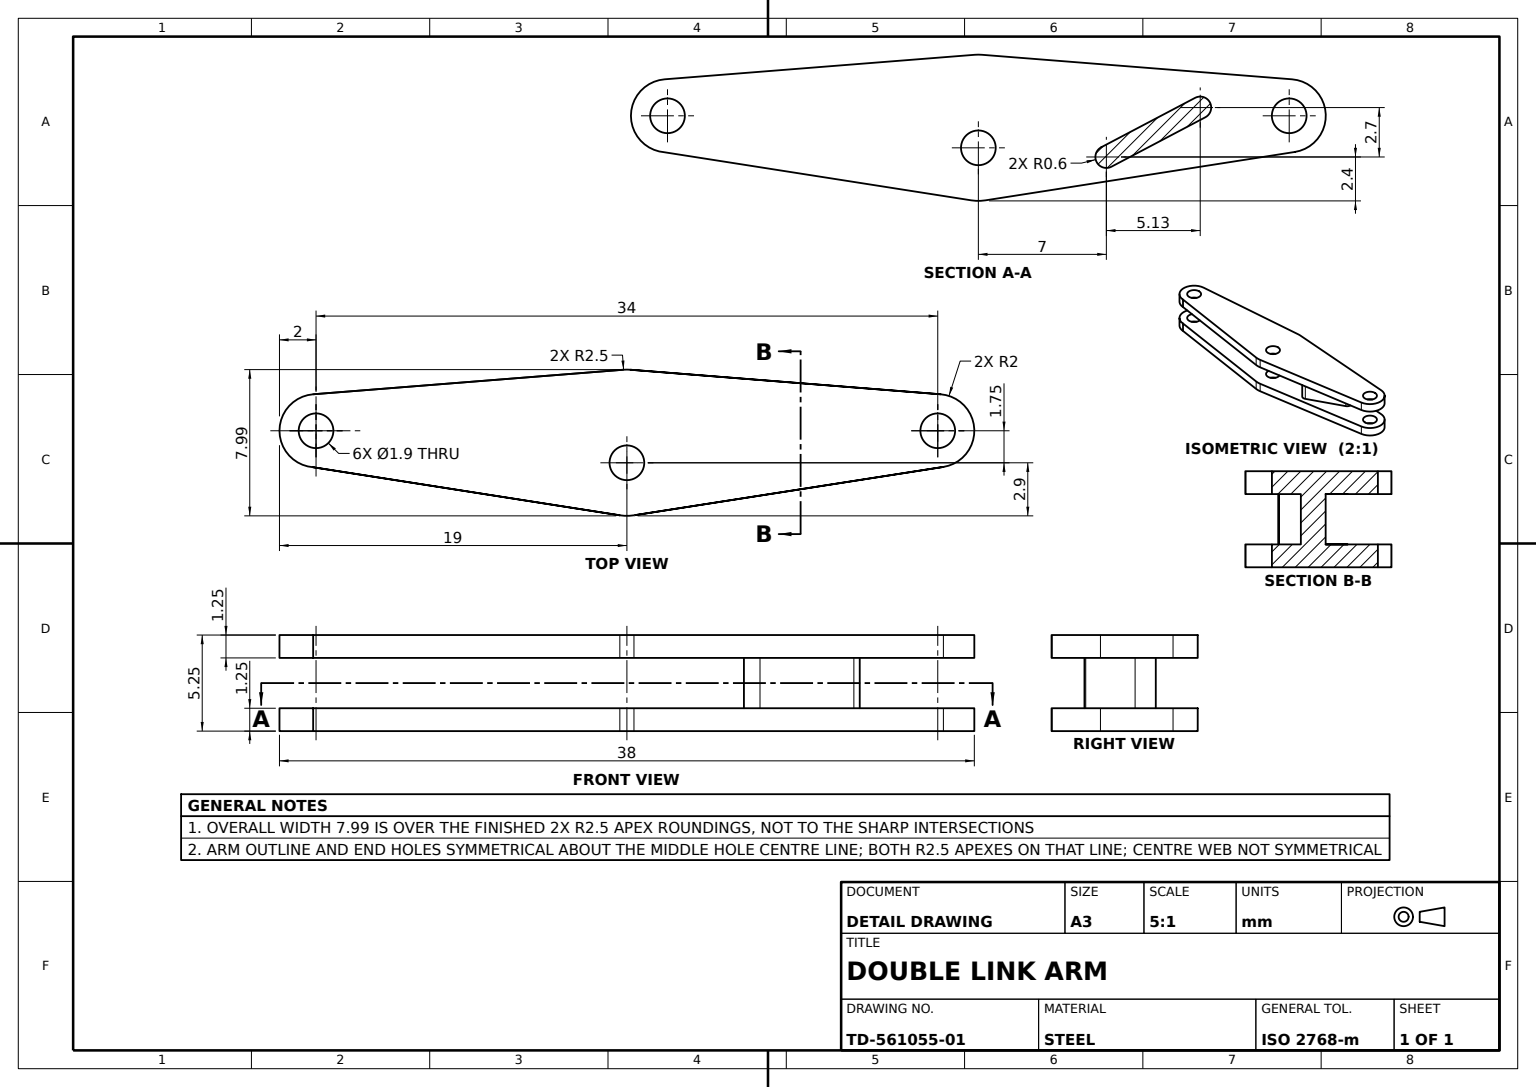
SolidWorks part; units mm, degrees
material "Plain Carbon Steel"
ref_plane "Front Plane" through (0, 0, 0) normal (0, 0, 1) x (1, 0, 0)
ref_plane "Top Plane" through (0, 0, 0) normal (0, 1, 0) x (1, 0, 0)
ref_plane "Right Plane" through (0, 0, 0) normal (1, 0, 0) x (0, 0, -1)
sketch "Arm Profile Sketch" plane through (0, 0, 0) normal (0, 1, 0) x (1, 0, 0)
  line L0 (17, 0) -> (-17, 0) construction
  line L1 (0, -4.65) -> (0, 3.35) construction
  line L2 (-17.1576, 1.9938) -> (-0.197, 3.3344)
  line L3 (-17.1576, -1.9938) -> (-0.3863, -4.6199)
  line L4 (0.197, 3.3344) -> (17.1576, 1.9938)
  line L5 (0.3863, -4.62) -> (17.3087, -1.976)
  circle A0 centre (-17, 0) radius 0.95
  arc A1 (-17.1576, 1.9938) -> (-17.1576, -1.9938) centre (-17, 0) ccw
  circle A2 centre (17, 0) radius 0.95
  arc A3 (17.3087, -1.976) -> (17.1576, 1.9938) centre (17, 0) ccw
  arc A4 (-0.3863, -4.6199) -> (0.3863, -4.62) centre (0.0004, -2.15) ccw
  arc A5 (0.197, 3.3344) -> (-0.197, 3.3344) centre (0, 0.8422) ccw
  circle A6 centre (0, -1.75) radius 0.95
  point P12 (0, -3.35)
  point P14 (0, 0)
  point P24 (0, -4.65)
  dimension "D3" = 8
  dimension "D4" = 4
  dimension "D5" = 1.9
  dimension "D6" = 4
  dimension "D7" = 1.9
  dimension "D8" = 2.5
  dimension "D9" = 1.9
  dimension "D1" = 34
  dimension "D2" = 3.35
  dimension "D10" = 1.75
extrude "Arm Body" add sketch "Arm Profile Sketch" along normal mid plane 5.25
sketch "Fork Slot Sketch" plane through (0, 0, 0) normal (0, 0, 1) x (1, 0, 0)
  line L0 (-17.1576, 2.625) -> (-0.3863, 2.625) construction
  line L1 (-19.5642, 1.375) -> (19.5642, 1.375)
  line L2 (-19.5642, 1.375) -> (-19.5642, -1.375)
  line L3 (-19.5642, -1.375) -> (19.5642, -1.375)
  line L4 (19.5642, 1.375) -> (19.5642, -1.375)
  line L5 (-19.5642, 1.375) -> (19.5642, -1.375) construction
  line L6 (-19.5642, -1.375) -> (19.5642, 1.375) construction
  point P0 (0, 0)
  dimension "D1" = 1.25
  dimension "D2" = 19.5642
extrude "Fork Slot Cut" cut sketch "Fork Slot Sketch" against normal mid plane 45.25
sketch "Centre Web Sketch" plane through (0, 0, 0) normal (0, 1, 0) x (1, 0, 0)
  line L0 (0, 0) -> (14.6106, 0) construction
  line L1 (0.3365, 0.45) -> (12.1332, 0.45) construction
  line L2 (7, -2.25) -> (12.1332, 0.45) construction
  line L3 (6.7207, -1.719) -> (11.8539, 0.981)
  line L4 (7.2793, -2.781) -> (12.4125, -0.081)
  arc A0 (6.7207, -1.719) -> (7.2793, -2.781) centre (7, -2.25) ccw
  arc A1 (12.4125, -0.081) -> (11.8539, 0.981) centre (12.1332, 0.45) ccw
  point P7 (9.5666, -0.9)
  dimension "D2" = 0.6
  dimension "D1" = 5.8
  dimension "D3" = 0.45
  dimension "D4" = 2.25
  dimension "D5" = 7
extrude "Centre Web" add sketch "Centre Web Sketch" along normal up to next (2.625 mm away) and the other way up to next (1.375 mm away)
